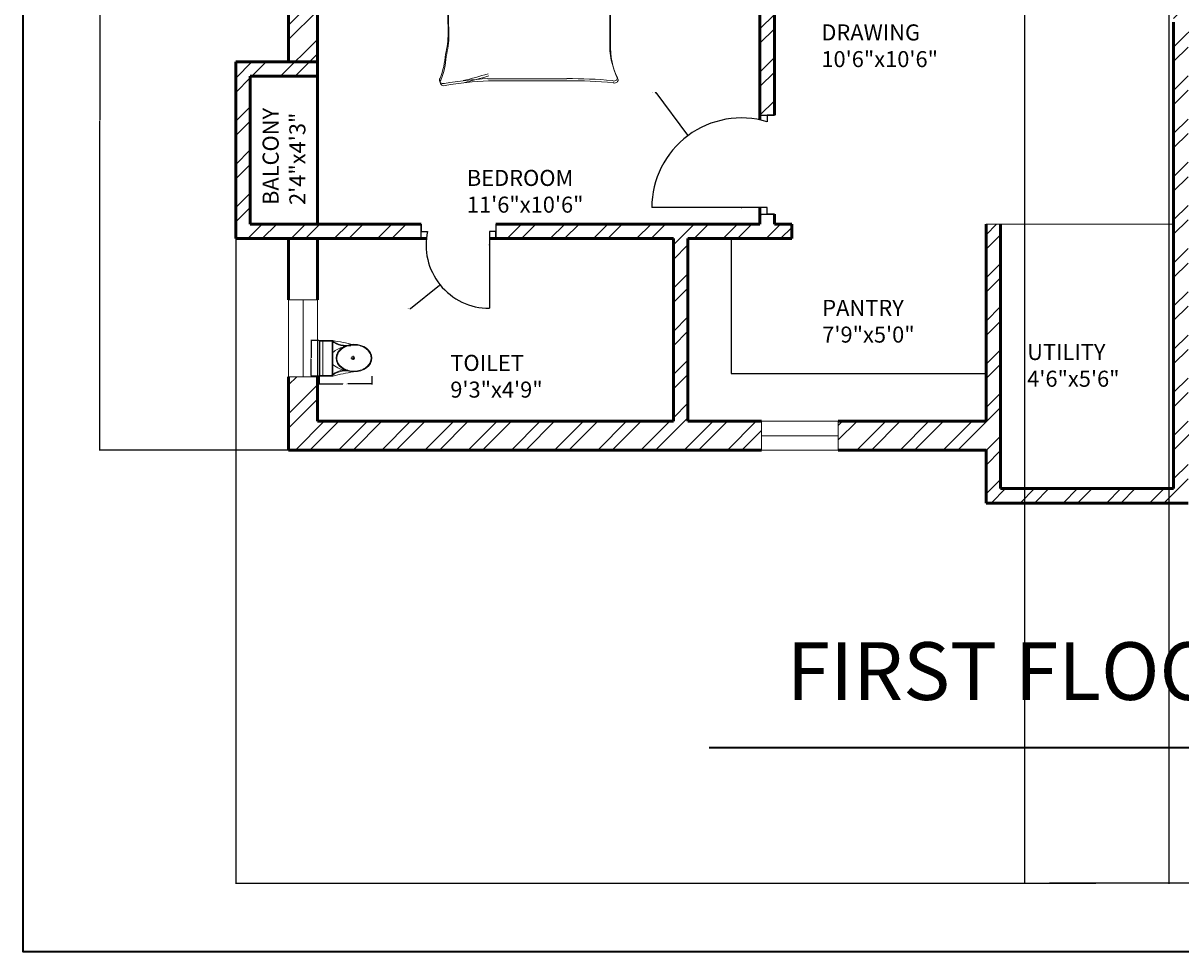
# Model space of a CAD drawing. Units: inches. Extents: x 1896 to 2572, y 1528 to 2474.
# Tile 1 of 10: x 1896 to 2257, y 1528 to 1818. Entities that reach past the tile are written whole.
import ezdxf

# ---------------------------------------------------------------- set-up
doc = ezdxf.new("R2010")
doc.units = ezdxf.units.IN
for name, color, linetype, lineweight in [('A-ANNO-DIMS', 2, 'Continuous', 18), ('A-ANNO-TTLB', 7, 'Continuous', 35), ('A-AREA-IDEN', 7, 'Continuous', 18), ('A-DOOR', 11, 'Continuous', 25), ('A-FLOR', 7, 'Continuous', 18), ('A-FLOR-CASE', 7, 'Continuous', 25), ('A-FLOR-FIXT', 8, 'Continuous', 18), ('A-FURN', 8, 'Continuous', 18), ('A-GLAZ', 131, 'Continuous', 20), ('A-WALL', 7, 'Continuous', 50)]:
    doc.layers.add(name, color=color, linetype=linetype, lineweight=lineweight)
doc.layers.add('A-WALL-PATT', color=215, linetype='Continuous', lineweight=13, true_color=0xa953a0)
doc.styles.get("Standard").update_dxf_attribs({"font": 'arial.ttf'})
doc.dimstyles.get("Standard").update_dxf_attribs({"dimtxt": 0.18, "dimasz": 0.18, "dimexe": 0.18, "dimexo": 0.0625, "dimgap": 0.09, "dimtad": 0, "dimtih": 1, "dimtoh": 1, "dimdec": 4, "dimzin": 0, "dimdsep": 46, "dimtxsty": 'Standard', "dimcen": 0.09, "dimadec": 0, "dimazin": 0, "dimtfac": 1, "dimtdec": 4, "dimtofl": 0, "dimtmove": 0, "dimatfit": 3, "dimfxl": 1, "dimtolj": 1, "dimtzin": 0, "dimarcsym": 0})

# ---------------------------------------------------------------- blocks, each defined once
blk = doc.blocks.new('A$C31115884')
for p, q in [((258, 466), (258, 523)), ((283, 498), (223, 498)), ((0, 200), (0, 0)), ((520, 200), (0, 200)), ((10, 190), (10, 10)), ((510, 190), (10, 190)), ((510, 10), (510, 190)), ((520, 0), (520, 200)), ((510, 54), (0, 54)), ((10, 10), (510, 10)), ((0, 0), (520, 0))]:
    blk.add_line(p, q)
blk.add_circle((256, 496), 23.6)
for centre, radius, start, end in [((2778, -205), 2807, 165.4549, 171.7133), ((-295, 403), 365, 324.2091, 9.3499), ((-295, 403), 375, 324.2091, 9.3499), ((384, 406), 293, 190.2774, 224.1564), ((139, 406), 293, 315.8436, 2.6563), ((806, 403), 375, 179.2036, 215.7909), ((806, 403), 365, 170.6501, 215.7909), ((3237, 905), 2807, 188.2867, 194.5451)]:
    blk.add_arc(centre, radius, start, end)
blk.add_ellipse((256, 510), major_axis=(0, -261), ratio=0.772727)
blk.add_open_spline([(256, 259), (263, 259), (270, 260), (288, 262), (299, 265), (320, 273), (330, 278), (350, 291), (360, 299), (378, 316), (386, 326), (402, 347), (409, 358), (421, 383), (427, 395), (436, 422), (440, 436), (445, 465), (447, 480), (448, 509), (448, 524), (445, 553), (443, 568), (436, 596), (432, 610), (422, 636), (416, 649), (402, 672), (395, 683), (379, 703), (370, 712), (351, 728), (341, 735), (321, 746), (310, 751), (289, 757), (278, 759), (256, 761), (245, 761), (223, 757), (212, 754), (191, 746), (181, 741), (161, 728), (151, 720), (133, 703), (125, 693), (110, 672), (103, 660), (90, 636), (85, 623), (76, 596), (72, 582), (67, 553), (66, 538), (64, 509), (65, 494), (68, 465), (70, 450), (77, 422), (81, 408), (91, 382), (97, 370), (111, 346), (118, 335), (135, 316), (144, 307), (162, 291), (172, 284), (193, 273), (203, 269), (225, 262), (236, 260), (250, 259), (253, 259), (256, 259)], degree=3, knots=[0, 0, 0, 0, 0.110105, 0.110105, 0.285049, 0.285049, 0.459994, 0.459994, 0.634938, 0.634938, 0.809882, 0.809882, 0.984827, 0.984827, 1.159771, 1.159771, 1.334715, 1.334715, 1.50966, 1.50966, 1.684604, 1.684604, 1.859549, 1.859549, 2.034493, 2.034493, 2.209437, 2.209437, 2.384382, 2.384382, 2.559326, 2.559326, 2.73427, 2.73427, 2.909215, 2.909215, 3.084159, 3.084159, 3.259103, 3.259103, 3.434048, 3.434048, 3.608992, 3.608992, 3.783936, 3.783936, 3.958881, 3.958881, 4.133825, 4.133825, 4.30877, 4.30877, 4.483714, 4.483714, 4.658658, 4.658658, 4.833603, 4.833603, 5.008547, 5.008547, 5.183491, 5.183491, 5.358436, 5.358436, 5.53338, 5.53338, 5.708324, 5.708324, 5.883269, 5.883269, 6.058213, 6.058213, 6.233158, 6.233158, 6.283185, 6.283185, 6.283185, 6.283185])
blk = doc.blocks.new('BED-DOUBLE')
for p, q in [((3.47, 63.33), (3.47, 81.44)), ((3.47, 63.33), (3.47, 81.44)), ((3.47, 81.44), (51.49, 81.44)), ((3.47, 79.91), (51.27, 79.91)), ((3.47, 79.91), (51.26, 79.91)), ((3.7, 62.69), (3.7, 80.8)), ((3.7, 62.69), (3.7, 80.8)), ((24.54, 78.99), (25.98, 79.57)), ((24.54, 78.99), (25.98, 79.57)), ((25.98, 79.57), (26.56, 74.22)), ((25.98, 79.57), (26.56, 74.22)), ((51.26, 81.44), (51.26, 54.83)), ((51.27, 81.44), (51.27, 54.83)), ((51.49, 81.44), (51.49, 80.8)), ((51.49, 80.8), (51.49, 54.19)), ((51.49, 80.8), (51.49, 54.19)), ((3.7, 79.27), (51.49, 79.27)), ((3.7, 79.27), (51.49, 79.27)), ((3.89, 78.13), (4.47, 74.95)), ((3.89, 78.13), (4.47, 74.95)), ((3.9, 78.11), (8.18, 78.43)), ((3.9, 78.11), (8.18, 78.43)), ((4.12, 77.49), (4.7, 74.31)), ((4.12, 77.49), (4.7, 74.31)), ((4.13, 77.47), (8.41, 77.8)), ((4.13, 77.47), (8.41, 77.8)), ((8.18, 78.43), (8.28, 78.42)), ((8.18, 78.43), (8.28, 78.42)), ((8.28, 78.42), (12.11, 78.13)), ((8.28, 78.42), (12.11, 78.13)), ((8.41, 77.8), (8.51, 77.78)), ((8.41, 77.8), (8.51, 77.78)), ((8.51, 77.78), (12.34, 77.49)), ((8.51, 77.78), (12.34, 77.49)), ((12.11, 78.13), (17.6, 77.12)), ((12.11, 78.13), (17.6, 77.12)), ((12.34, 77.49), (17.83, 76.48)), ((12.34, 77.49), (17.83, 76.48)), ((14.85, 77.69), (16.88, 78.42)), ((14.85, 77.69), (16.88, 78.42)), ((15.08, 77.05), (17.11, 77.78)), ((15.08, 77.05), (17.11, 77.78)), ((16.88, 78.42), (19.77, 79.14)), ((16.88, 78.42), (19.77, 79.14)), ((17.11, 77.78), (20, 78.5)), ((17.11, 77.78), (20, 78.5)), ((19.77, 79.14), (20.09, 79.14)), ((19.77, 79.14), (20.09, 79.14)), ((20, 78.5), (20.32, 78.5)), ((20, 78.5), (20.32, 78.5)), ((20.09, 79.14), (24.54, 78.99)), ((20.09, 79.14), (24.54, 78.99)), ((20.32, 78.5), (24.77, 78.36)), ((20.32, 78.5), (24.76, 78.36)), ((24.76, 78.36), (26.21, 78.93)), ((24.77, 78.36), (26.21, 78.93)), ((26.21, 78.93), (26.79, 73.58)), ((26.21, 78.93), (26.79, 73.58)), ((27.98, 78.95), (27.73, 73.58)), ((27.98, 78.95), (27.73, 73.58)), ((28.21, 78.31), (27.96, 72.94)), ((28.2, 78.31), (27.96, 72.94)), ((29.46, 78.46), (27.98, 78.95)), ((29.46, 78.46), (27.98, 78.95)), ((29.68, 77.83), (28.2, 78.31)), ((29.68, 77.83), (28.21, 78.31)), ((33.88, 78.89), (29.46, 78.46)), ((33.88, 78.89), (29.46, 78.46)), ((34.11, 78.25), (29.68, 77.83)), ((34.11, 78.25), (29.68, 77.83)), ((34.2, 78.91), (33.88, 78.89)), ((34.2, 78.91), (33.88, 78.89)), ((34.43, 78.27), (34.11, 78.25)), ((34.43, 78.27), (34.11, 78.25)), ((37.14, 78.37), (34.2, 78.91)), ((37.13, 78.37), (34.2, 78.91)), ((37.36, 77.73), (34.43, 78.27)), ((37.36, 77.73), (34.43, 78.27)), ((41.91, 78.37), (36.49, 77.02)), ((41.91, 78.37), (36.49, 77.02)), ((42.14, 77.73), (36.72, 76.38)), ((42.14, 77.73), (36.72, 76.38)), ((39.2, 77.77), (37.13, 78.37)), ((39.2, 77.77), (37.14, 78.37)), ((39.43, 77.13), (37.36, 77.73)), ((39.43, 77.13), (37.36, 77.73)), ((45.71, 78.9), (41.91, 78.37)), ((45.71, 78.9), (41.91, 78.37)), ((45.94, 78.26), (42.14, 77.73)), ((45.94, 78.26), (42.14, 77.73)), ((50.11, 78.89), (44.71, 78.98)), ((44.71, 78.98), (45.71, 78.9)), ((50.11, 78.89), (44.71, 78.98)), ((44.71, 78.98), (45.71, 78.9)), ((50.34, 78.25), (44.94, 78.34)), ((44.94, 78.34), (45.94, 78.26)), ((50.34, 78.25), (44.94, 78.34)), ((44.94, 78.34), (45.94, 78.26)), ((49.31, 73.19), (48.13, 75.87)), ((49.31, 73.19), (48.13, 75.87)), ((50.11, 78.89), (49.73, 75.68)), ((50.11, 78.89), (49.73, 75.68)), ((50.34, 78.25), (49.96, 75.04)), ((50.34, 78.25), (49.96, 75.04)), ((4.47, 74.95), (4.04, 72.34)), ((4.47, 74.95), (4.04, 72.34)), ((4.04, 72.34), (4.62, 71.33)), ((4.04, 72.34), (4.62, 71.33)), ((4.7, 74.31), (4.27, 71.7)), ((4.7, 74.31), (4.27, 71.7)), ((4.47, 68.87), (5.05, 72.49)), ((4.47, 68.87), (5.05, 72.49)), ((5.05, 72.49), (6.06, 75.24)), ((5.05, 72.49), (6.06, 75.24)), ((5.28, 71.85), (6.29, 74.6)), ((5.28, 71.85), (6.29, 74.6)), ((26.56, 74.22), (27.14, 71.04)), ((26.56, 74.22), (27.14, 71.04)), ((26.79, 73.58), (27.37, 70.4)), ((26.79, 73.58), (27.37, 70.4)), ((27.73, 73.58), (27.35, 70.37)), ((27.73, 73.58), (27.35, 70.37)), ((27.96, 72.94), (27.58, 69.73)), ((27.96, 72.94), (27.58, 69.73)), ((49.54, 72.55), (48.36, 75.23)), ((49.54, 72.55), (48.36, 75.23)), ((50.11, 69.61), (49.31, 73.19)), ((50.11, 69.61), (49.31, 73.19)), ((50.34, 68.98), (49.54, 72.55)), ((50.34, 68.98), (49.54, 72.55)), ((49.73, 75.68), (50.33, 73.11)), ((49.73, 75.68), (50.33, 73.11)), ((50.33, 73.11), (49.81, 72.06)), ((50.33, 73.11), (49.81, 72.06)), ((49.96, 75.04), (50.56, 72.47)), ((49.96, 75.04), (50.56, 72.47)), ((50.56, 72.47), (50.04, 71.42)), ((50.56, 72.47), (50.04, 71.42)), ((4.27, 71.7), (4.85, 70.69)), ((4.27, 71.7), (4.85, 70.69)), ((4.76, 67.28), (4.47, 68.87)), ((4.76, 67.28), (4.47, 68.87)), ((4.7, 68.23), (5.28, 71.85)), ((4.7, 68.23), (5.28, 71.85)), ((27.14, 69.74), (26.56, 67.86)), ((27.14, 69.74), (26.56, 67.86)), ((27.37, 69.1), (26.79, 67.22)), ((27.37, 69.1), (26.79, 67.22)), ((27.14, 71.04), (27.14, 69.74)), ((27.14, 71.04), (27.14, 69.74)), ((27.35, 70.37), (27.44, 69.07)), ((27.35, 70.37), (27.44, 69.07)), ((27.37, 70.4), (27.37, 69.1)), ((27.37, 70.4), (27.37, 69.1)), ((27.44, 69.07), (28.13, 67.23)), ((27.44, 69.07), (28.13, 67.23)), ((27.58, 69.73), (27.66, 68.43)), ((27.58, 69.73), (27.66, 68.43)), ((49.92, 68.01), (50.11, 69.61)), ((49.92, 68.01), (50.11, 69.61)), ((50.15, 67.37), (50.34, 68.98)), ((50.15, 67.37), (50.34, 68.98)), ((4.18, 64.1), (4.76, 67.28)), ((4.18, 64.1), (4.76, 67.28)), ((4.41, 63.46), (4.99, 66.64)), ((4.41, 63.46), (4.99, 66.64)), ((4.99, 66.64), (4.7, 68.23)), ((4.99, 66.64), (4.7, 68.23)), ((6.38, 65.81), (10.41, 65.15)), ((6.38, 65.81), (10.41, 65.15)), ((6.61, 65.18), (10.64, 64.51)), ((6.61, 65.18), (10.64, 64.51)), ((10.41, 65.15), (9.28, 64.83)), ((10.41, 65.15), (9.28, 64.83)), ((10.41, 65.15), (17.42, 64.72)), ((10.41, 65.15), (17.42, 64.72)), ((17.42, 64.72), (19.38, 65.27)), ((17.42, 64.72), (19.38, 65.27)), ((19.38, 65.27), (24.52, 64.87)), ((19.38, 65.27), (24.52, 64.87)), ((24.1, 65.18), (20.96, 66.27)), ((24.1, 65.18), (20.96, 66.27)), ((24.33, 64.54), (21.19, 65.63)), ((24.33, 64.54), (21.19, 65.63)), ((26.56, 65.18), (24.1, 65.18)), ((26.56, 65.18), (24.1, 65.18)), ((26.56, 67.86), (26.56, 65.18)), ((26.56, 67.86), (26.56, 65.18)), ((26.79, 67.22), (26.79, 64.54)), ((26.79, 67.22), (26.79, 64.54)), ((27.66, 68.43), (28.36, 66.59)), ((27.66, 68.43), (28.36, 66.59)), ((28.13, 67.23), (28.3, 64.55)), ((28.13, 67.23), (28.3, 64.55)), ((28.36, 66.59), (28.53, 63.91)), ((28.36, 66.59), (28.53, 63.91)), ((30.75, 64.7), (33.82, 65.99)), ((30.75, 64.7), (33.82, 65.99)), ((30.98, 64.06), (34.05, 65.35)), ((30.98, 64.06), (34.05, 65.35)), ((32.56, 65.81), (36.6, 65.15)), ((32.56, 65.81), (36.6, 65.15)), ((32.79, 65.18), (36.82, 64.51)), ((32.79, 65.18), (36.82, 64.51)), ((36.6, 65.15), (43.61, 64.72)), ((36.6, 65.15), (43.61, 64.72)), ((43.61, 64.72), (45.57, 65.27)), ((43.61, 64.72), (45.57, 65.27)), ((45.57, 65.27), (50.7, 64.87)), ((45.57, 65.27), (50.7, 64.87)), ((50.7, 64.87), (49.92, 68.01)), ((50.7, 64.87), (49.92, 68.01)), ((50.93, 64.23), (50.15, 67.37)), ((50.93, 64.23), (50.15, 67.37)), ((9.28, 64.83), (4.18, 64.1)), ((9.28, 64.83), (4.18, 64.1)), ((9.51, 64.19), (4.41, 63.46)), ((9.51, 64.19), (4.41, 63.46)), ((10.64, 64.51), (9.51, 64.19)), ((10.64, 64.51), (9.51, 64.19)), ((10.64, 64.51), (17.65, 64.08)), ((10.64, 64.51), (17.65, 64.08)), ((17.65, 64.08), (19.61, 64.63)), ((17.65, 64.08), (19.61, 64.63)), ((19.61, 64.63), (24.74, 64.23)), ((19.61, 64.63), (24.74, 64.23)), ((26.79, 64.54), (24.33, 64.54)), ((26.79, 64.54), (24.33, 64.54)), ((28.3, 64.55), (30.75, 64.7)), ((28.3, 64.55), (30.75, 64.7)), ((28.53, 63.91), (30.98, 64.06)), ((28.53, 63.91), (30.98, 64.06)), ((30.26, 64.06), (34.45, 57.57)), ((30.26, 64.06), (34.45, 57.57)), ((30.49, 63.42), (34.68, 56.93)), ((30.49, 63.42), (34.68, 56.93)), ((40.64, 61.13), (32.31, 64.06)), ((40.64, 61.13), (32.31, 64.06)), ((40.87, 60.49), (32.53, 63.42)), ((40.87, 60.49), (32.53, 63.42)), ((36.82, 64.51), (43.83, 64.08)), ((36.82, 64.51), (43.83, 64.08)), ((43.83, 64.08), (45.79, 64.63)), ((43.83, 64.08), (45.79, 64.63)), ((45.79, 64.63), (50.93, 64.23)), ((45.79, 64.63), (50.93, 64.23)), ((46.22, 59.11), (40.64, 61.13)), ((46.22, 59.11), (40.64, 61.13)), ((46.45, 58.48), (40.87, 60.49)), ((46.45, 58.48), (40.87, 60.49)), ((49.16, 56.95), (46.22, 59.11)), ((49.16, 56.95), (46.22, 59.11)), ((49.39, 56.31), (46.45, 58.48)), ((49.39, 56.31), (46.45, 58.48)), ((34.45, 57.57), (36.15, 53.08)), ((34.45, 57.57), (36.15, 53.08)), ((34.68, 56.93), (36.38, 52.44)), ((34.68, 56.93), (36.38, 52.44)), ((52.87, 53.7), (49.16, 56.95)), ((52.87, 53.7), (49.16, 56.95)), ((53.1, 53.06), (49.39, 56.31)), ((53.1, 53.06), (49.39, 56.31)), ((36.15, 53.08), (36.46, 51.07)), ((36.15, 53.08), (36.46, 51.07)), ((36.38, 52.44), (36.69, 50.43)), ((36.38, 52.44), (36.69, 50.43)), ((36.46, 51.07), (38.94, 51.69)), ((36.46, 51.07), (38.94, 51.69)), ((36.69, 50.43), (39.17, 51.05)), ((36.69, 50.43), (39.17, 51.05)), ((38.94, 51.69), (40.95, 52.61)), ((38.94, 51.69), (40.95, 52.61)), ((39.17, 51.05), (41.18, 51.97)), ((39.17, 51.05), (41.18, 51.97)), ((40.95, 52.61), (44.36, 53.08)), ((40.95, 52.61), (44.36, 53.08)), ((41.18, 51.97), (44.59, 52.44)), ((41.18, 51.97), (44.59, 52.44)), ((44.36, 53.08), (48.23, 53.39)), ((44.36, 53.08), (48.23, 53.39)), ((44.59, 52.44), (48.46, 52.75)), ((44.59, 52.44), (48.46, 52.75)), ((48.23, 53.39), (51.33, 53.08)), ((48.23, 53.39), (51.33, 53.08)), ((48.46, 52.75), (51.56, 52.44)), ((48.46, 52.75), (51.56, 52.44)), ((51.33, 53.08), (52.87, 53.7)), ((51.33, 53.08), (52.87, 53.7)), ((51.56, 52.44), (53.1, 53.06)), ((51.56, 52.44), (53.1, 53.06)), ((52.95, 51.95), (52.87, 53.7, 3.87)), ((52.95, 51.95), (52.87, 53.7, 3.87)), ((53.18, 51.31), (53.1, 53.06, 3.87)), ((53.17, 51.31), (53.1, 53.06, 3.87)), ((15.06, 2.2), (39.68, 2.2)), ((15.06, 2.2), (39.68, 2.2)), ((15.29, 1.56), (39.91, 1.56)), ((15.29, 1.56), (39.91, 1.56))]:
    blk.add_line(p, q)
for centre, radius, start, end in [((85.16, 61.35), 83.31, 178.7218, 185.604), ((85.16, 61.35), 83.31, 178.7218, 185.604), ((21.36, -100.61), 164.97, 86.0865, 96.7821), ((21.36, -100.61), 164.97, 86.0865, 96.7821), ((85.39, 60.71), 83.31, 178.7218, 185.604), ((85.39, 60.71), 83.31, 178.7218, 185.604), ((21.59, -101.25), 164.97, 86.0865, 96.7821), ((21.59, -101.25), 164.97, 86.0865, 96.7821), ((17.76, -74.87), 129.02, 81.7845, 96.9006), ((17.76, -74.87), 129.02, 81.7845, 96.9006), ((17.98, -75.51), 129.02, 81.7845, 96.9006), ((17.98, -75.51), 129.02, 81.7845, 96.9006), ((-167.31, 50.27), 170.11, 358.4762, 1.0082), ((-167.31, 50.27), 170.11, 358.4762, 1.0082), ((-167.08, 49.63), 170.11, 358.4762, 1.0082), ((-167.08, 49.63), 170.11, 358.4762, 1.0082), ((36.64, 51), 0.185, 160.2464, 271.1377), ((36.64, 51), 0.185, 160.2464, 271.1377), ((31.15, 79.96), 29.65, 280.6617, 289.8806), ((31.15, 79.96), 29.65, 280.6617, 289.8806), ((31.38, 79.32), 29.65, 280.6617, 289.8806), ((31.38, 79.32), 29.65, 280.6617, 289.8806), ((43.74, 46.38), 6.22, 78.6608, 113.7384), ((43.74, 46.38), 6.22, 78.6608, 113.7384), ((43.97, 45.74), 6.22, 78.6608, 113.7384), ((43.97, 45.74), 6.22, 78.6608, 113.7384), ((51.33, 88.1), 36.18, 259.8763, 272.5657), ((51.33, 88.1), 36.18, 259.8763, 272.5657), ((51.56, 87.46), 36.18, 259.8763, 272.5657), ((51.56, 87.46), 36.18, 259.8763, 272.5657), ((182.27, 45.13), 129.5, 176.9791, 183.8365), ((182.27, 45.13), 129.5, 176.9791, 183.8365), ((182.49, 44.49), 129.5, 176.9791, 183.8365), ((182.49, 44.49), 129.5, 176.9791, 183.8365), ((36.86, 50.36), 0.185, 160.2464, 271.1377), ((36.86, 50.36), 0.185, 160.2464, 271.1377), ((484.82, 30.83), 482.31, 178.2277, 181.7185), ((484.82, 30.83), 482.31, 178.2277, 181.7185), ((485.05, 30.19), 482.31, 178.2277, 181.7185), ((485.05, 30.19), 482.31, 178.2277, 181.7185), ((-4508.74, 13.62), 4561.86, 0.00217, 0.28689), ((-4508.74, 13.62), 4561.86, 0.00217, 0.28689), ((-4508.52, 12.98), 4561.86, 0.00217, 0.28689), ((-4508.52, 12.98), 4561.86, 0.00217, 0.28689), ((-26.9, 16.93), 29.63, 346.0648, 358.9113), ((-26.9, 16.93), 29.63, 346.0648, 358.9113), ((-26.67, 16.29), 29.63, 346.0648, 358.9113), ((-26.67, 16.29), 29.63, 346.0648, 358.9113), ((76.16, 12.78), 23.07, 177.4714, 206.4681), ((76.16, 12.78), 23.07, 177.4714, 206.4681), ((76.39, 12.14), 23.07, 177.4714, 206.4681), ((76.39, 12.14), 23.07, 177.4714, 206.4681), ((-21.66, 11.17), 23.56, 337.9751, 356.652), ((-21.66, 11.17), 23.56, 337.9751, 356.652), ((-21.43, 10.53), 23.56, 337.9751, 356.652), ((-21.43, 10.53), 23.56, 337.9751, 356.652), ((-17.22, 105.16), 106.46, 283.3832, 287.7053), ((-17.22, 105.16), 106.46, 283.3832, 287.7053), ((1.09, 1.73), 1.09, 146.1736, 293.4781), ((1.09, 1.73), 1.09, 146.1736, 293.4781), ((1.32, 1.09), 1.09, 146.1736, 293.4781), ((1.32, 1.09), 1.09, 146.1736, 293.4781), ((21.43, -119.39), 121.76, 92.9958, 99.4091), ((21.43, -119.39), 121.76, 92.9958, 99.4091), ((21.65, -120.03), 121.76, 92.9958, 99.4091), ((21.65, -120.03), 121.76, 92.9958, 99.4091), ((-16.99, 104.52), 106.46, 283.3832, 287.7053), ((-16.99, 104.52), 106.46, 283.3832, 287.7053), ((41.15, -130.83), 133.04, 84.4998, 90.6351), ((41.15, -130.83), 133.04, 84.4998, 90.6351), ((41.38, -131.47), 133.04, 84.4998, 90.6351), ((41.38, -131.47), 133.04, 84.4998, 90.6351), ((54.41, 2.57), 1.1, 242.6588, 356.02), ((54.41, 2.57), 1.1, 242.6588, 356.02), ((54.64, 1.93), 1.1, 242.6588, 356.02), ((54.64, 1.93), 1.1, 242.6588, 356.02)]:
    blk.add_arc(centre, radius, start, end)
blk = doc.blocks.new('WIN-24IN')
for p, q in [((4.5, 24), (0, 24)), ((0, 24), (9, 24)), ((0, 24), (0, 0)), ((4.5, 0), (4.5, 24)), ((9, 0), (9, 24)), ((0, 0), (9, 0)), ((9, 0), (4.5, 0))]:
    blk.add_line(p, q)
blk = doc.blocks.new('*D9')
at = {"layer": 'A-ANNO-DIMS', "color": 0, "lineweight": -2, "transparency": 16777216}
for p, q in [((1988.15, 1707.44), (1988.15, 1704.86)), ((1988.33, 1705.04), (1995.58, 1705.04)), ((2004.37, 1705.04), (1997.13, 1705.04)), ((2004.55, 1707.44), (2004.55, 1704.86))]:
    blk.add_line(p, q, dxfattribs=at)
at = {"layer": 'A-ANNO-DIMS', "color": 0, "transparency": 16777216}
for points in [[(1988.33, 1705.07), (1988.33, 1705.01), (1988.15, 1705.04)], [(2004.37, 1705.07), (2004.37, 1705.01), (2004.55, 1705.04)]]:
    blk.add_solid(points, dxfattribs=at)
at = {"layer": 'Defpoints', "color": 0, "transparency": 16777216}
for p in [(1988.15, 1707.5), (2004.55, 1707.5), (2004.55, 1705.04)]:
    blk.add_point(p, dxfattribs=at)
at = {"layer": 'A-ANNO-DIMS', "color": 0, "transparency": 16777216, "insert": (1996.35, 1705.04), "char_height": 0.18, "attachment_point": 5}
blk.add_mtext('\\A1;WC 16 TYP.', dxfattribs=at)
blk = doc.blocks.new('*D10')
at = {"layer": 'A-ANNO-DIMS', "color": 0, "lineweight": -2, "transparency": 16777216}
for p, q in [((1988.09, 1718.57), (1985.51, 1718.57)), ((1985.69, 1718.39), (1985.69, 1713.22)), ((1985.69, 1707.68), (1985.69, 1712.86)), ((1988.09, 1707.5), (1985.51, 1707.5))]:
    blk.add_line(p, q, dxfattribs=at)
at = {"layer": 'A-ANNO-DIMS', "color": 0, "transparency": 16777216}
for points in [[(1985.66, 1718.39), (1985.72, 1718.39), (1985.69, 1718.57)], [(1985.66, 1707.68), (1985.72, 1707.68), (1985.69, 1707.5)]]:
    blk.add_solid(points, dxfattribs=at)
at = {"layer": 'Defpoints', "color": 0, "transparency": 16777216}
for p in [(1988.15, 1718.57), (1985.69, 1707.5), (1988.15, 1707.5)]:
    blk.add_point(p, dxfattribs=at)
at = {"layer": 'A-ANNO-DIMS', "color": 0, "transparency": 16777216, "insert": (1985.69, 1713.04), "char_height": 0.18, "attachment_point": 5}
blk.add_mtext('\\A1;11 TYP.', dxfattribs=at)
blk = doc.blocks.new('*D19')
at = {"layer": 'A-ANNO-DIMS', "color": 0, "lineweight": -2, "transparency": 16777216}
for p, q in [((2469.12, 1813.34), (2469.12, 1549.1)), ((1962.12, 1750.34), (1962.12, 1549.1)), ((1962.3, 1549.28), (2215.33, 1549.28)), ((2468.94, 1549.28), (2215.91, 1549.28))]:
    blk.add_line(p, q, dxfattribs=at)
at = {"layer": 'A-ANNO-DIMS', "color": 0, "transparency": 16777216}
for points in [[(1962.3, 1549.31), (1962.3, 1549.25), (1962.12, 1549.28)], [(2468.94, 1549.31), (2468.94, 1549.25), (2469.12, 1549.28)]]:
    blk.add_solid(points, dxfattribs=at)
at = {"layer": 'Defpoints', "color": 0, "transparency": 16777216}
for p in [(2469.12, 1813.4), (1962.12, 1750.4), (2469.12, 1549.28)]:
    blk.add_point(p, dxfattribs=at)
at = {"layer": 'A-ANNO-DIMS', "color": 0, "transparency": 16777216, "insert": (2215.62, 1549.28), "char_height": 0.18, "attachment_point": 5}
blk.add_mtext('\\A1;507', dxfattribs=at)
blk = doc.blocks.new('*D20')
at = {"layer": 'A-ANNO-DIMS', "color": 0, "lineweight": -2, "transparency": 16777216}
for p, q in [((2180.68, 2431.4), (2511.65, 2431.4)), ((2511.47, 2431.22), (2511.47, 2049.83)), ((2511.47, 1668.08), (2511.47, 2049.47)), ((2452.68, 1667.9), (2511.65, 1667.9))]:
    blk.add_line(p, q, dxfattribs=at)
at = {"layer": 'A-ANNO-DIMS', "color": 0, "transparency": 16777216}
for points in [[(2511.44, 2431.22), (2511.5, 2431.22), (2511.47, 2431.4)], [(2511.44, 1668.08), (2511.5, 1668.08), (2511.47, 1667.9)]]:
    blk.add_solid(points, dxfattribs=at)
at = {"layer": 'Defpoints', "color": 0, "transparency": 16777216}
for p in [(2180.62, 2431.4), (2511.47, 2431.4), (2452.62, 1667.9)]:
    blk.add_point(p, dxfattribs=at)
at = {"layer": 'A-ANNO-DIMS', "color": 0, "transparency": 16777216, "insert": (2511.47, 2049.65), "char_height": 0.18, "attachment_point": 5}
blk.add_mtext('\\A1;763.5', dxfattribs=at)
blk = doc.blocks.new('*D28')
at = {"layer": 'A-ANNO-DIMS', "color": 0, "lineweight": -2, "transparency": 16777216}
for p, q in [((1987.56, 1889.9), (1919.59, 1889.9)), ((1919.77, 1889.72), (1919.77, 1787.33)), ((1919.77, 1684.58), (1919.77, 1786.97)), ((1978.56, 1684.4), (1919.59, 1684.4))]:
    blk.add_line(p, q, dxfattribs=at)
at = {"layer": 'A-ANNO-DIMS', "color": 0, "transparency": 16777216}
for points in [[(1919.74, 1889.72), (1919.8, 1889.72), (1919.77, 1889.9)], [(1919.74, 1684.58), (1919.8, 1684.58), (1919.77, 1684.4)]]:
    blk.add_solid(points, dxfattribs=at)
at = {"layer": 'Defpoints', "color": 0, "transparency": 16777216}
for p in [(1987.62, 1889.9), (1919.77, 1684.4), (1978.62, 1684.4)]:
    blk.add_point(p, dxfattribs=at)
at = {"layer": 'A-ANNO-DIMS', "color": 0, "transparency": 16777216, "insert": (1919.77, 1787.15), "char_height": 0.18, "attachment_point": 5}
blk.add_mtext('\\A1;205.5', dxfattribs=at)
blk = doc.blocks.new('*D33')
at = {"layer": 'A-ANNO-DIMS', "color": 0, "lineweight": -2, "transparency": 16777216}
for p, q in [((2208.12, 2166.84), (2208.12, 1549.1)), ((2253.12, 2166.84), (2253.12, 1549.1)), ((2208.3, 1549.28), (2230.4, 1549.28)), ((2252.94, 1549.28), (2230.85, 1549.28))]:
    blk.add_line(p, q, dxfattribs=at)
at = {"layer": 'A-ANNO-DIMS', "color": 0, "transparency": 16777216}
for points in [[(2208.3, 1549.31), (2208.3, 1549.25), (2208.12, 1549.28)], [(2252.94, 1549.31), (2252.94, 1549.25), (2253.12, 1549.28)]]:
    blk.add_solid(points, dxfattribs=at)
at = {"layer": 'Defpoints', "color": 0, "transparency": 16777216}
for p in [(2208.12, 2166.9), (2253.12, 2166.9), (2253.12, 1549.28)]:
    blk.add_point(p, dxfattribs=at)
at = {"layer": 'A-ANNO-DIMS', "color": 0, "transparency": 16777216, "insert": (2230.62, 1549.28), "char_height": 0.18, "attachment_point": 5}
blk.add_mtext('\\A1;45', dxfattribs=at)
blk = doc.blocks.new('*D39')
at = {"layer": 'A-ANNO-DIMS', "color": 0, "lineweight": -2, "transparency": 16777216}
for p, q in [((2092.94, 1795.95), (2093.12, 1795.95)), ((2093.12, 1795.95), (2103.04, 1782.64)), ((2119.75, 1760.05), (2119.93, 1760.05)), ((2119.84, 1759.96), (2119.84, 1760.14))]:
    blk.add_line(p, q, dxfattribs=at)
at = {"layer": 'A-ANNO-DIMS', "color": 0, "transparency": 16777216}
blk.add_solid([(2103.06, 1782.65), (2103.01, 1782.62), (2103.14, 1782.49)], dxfattribs=at)
at = {"layer": 'Defpoints', "color": 0, "transparency": 16777216}
for p in [(2103.14, 1782.49), (2119.84, 1760.05)]:
    blk.add_point(p, dxfattribs=at)
at = {"layer": 'A-ANNO-DIMS', "color": 0, "transparency": 16777216, "insert": (2092.46, 1795.95), "char_height": 0.18, "attachment_point": 5}
blk.add_mtext('\\A1;R27.97', dxfattribs=at)
blk = doc.blocks.new('*D46')
at = {"layer": 'A-ANNO-DIMS', "color": 0, "lineweight": -2, "transparency": 16777216}
for p, q in [((2041.14, 1748.41), (2041.32, 1748.41)), ((2041.23, 1748.32), (2041.23, 1748.5)), ((2016.59, 1728.6), (2025.69, 1735.91)), ((2016.41, 1728.6), (2016.59, 1728.6))]:
    blk.add_line(p, q, dxfattribs=at)
at = {"layer": 'A-ANNO-DIMS', "color": 0, "transparency": 16777216}
blk.add_solid([(2025.67, 1735.94), (2025.71, 1735.89), (2025.83, 1736.02)], dxfattribs=at)
at = {"layer": 'Defpoints', "color": 0, "transparency": 16777216}
for p in [(2041.23, 1748.41), (2025.83, 1736.02)]:
    blk.add_point(p, dxfattribs=at)
at = {"layer": 'A-ANNO-DIMS', "color": 0, "transparency": 16777216, "insert": (2015.93, 1728.6), "char_height": 0.18, "attachment_point": 5}
blk.add_mtext('\\A1;R19.76', dxfattribs=at)

msp = doc.modelspace()

# ---------------------------------------------------------------- hatches: boundary and pattern name
at = {"layer": 'A-WALL-PATT'}
h = msp.add_hatch(dxfattribs=at)
h.set_pattern_fill('ANSI32', color=256)
h.paths.add_polyline_path([(2071.6224, 2382.3979), (2071.6224, 2422.3979), (2110.6224, 2422.3979), (2110.6224, 2382.3979), (2110.6224, 2357.5961), (2119.6224, 2357.5961), (2119.6224, 2422.3979), (2171.6224, 2422.3979), (2171.6224, 2373.3979), (2193.5093, 2373.3979), (2193.5093, 2377.8979), (2193.5093, 2382.3979), (2180.6224, 2382.3979), (2180.6224, 2431.3979), (2171.6224, 2431.3979), (2119.6224, 2431.3979), (2110.6224, 2431.3979), (2062.6224, 2431.3979), (2062.6224, 2422.3979), (2062.6224, 2382.3979), (1978.6224, 2382.3979), (1978.6224, 2313.0337), (1987.6224, 2313.0337), (1987.6224, 2373.3979), (2062.6224, 2373.3979), (2067.1224, 2373.3979), (2067.1224, 2353.7982), (2071.6224, 2353.8883)])
h.paths.add_polyline_path([(2287.4624, 2382.3979), (2229.5093, 2382.3979), (2229.5093, 2373.3979), (2253.1224, 2373.3979), (2253.1224, 2175.8979), (2247.1039, 2175.8979), (2247.1039, 2166.8979), (2253.1224, 2166.8979), (2253.1224, 2150.8283), (2262.1224, 2150.8283), (2262.1224, 2166.8979), (2262.1224, 2236.8979), (2349.0731, 2236.8979), (2349.0731, 2239.1479), (2349.0731, 2241.3979), (2262.1224, 2241.3979), (2262.1224, 2373.3979), (2287.4624, 2373.3979)])
h.paths.add_polyline_path([(2452.6224, 2382.3979), (2347.4624, 2382.3979), (2347.4624, 2373.3979), (2382.1224, 2373.3979), (2382.1224, 2334.0335), (2386.6224, 2334.0335), (2386.6224, 2373.3979), (2443.6224, 2373.3979), (2443.6224, 2316.2056), (2452.6224, 2316.2056)])
h.paths.add_polyline_path([(2452.6224, 2292.2056), (2448.1224, 2292.2056), (2443.6224, 2292.2056), (2443.6224, 2292.0047), (2443.6224, 2280.9372), (2443.6224, 2268.3979), (2386.6224, 2268.3979), (2386.6224, 2312.4044), (2384.3724, 2312.4044), (2382.1224, 2312.4044), (2382.1224, 2241.3979), (2379.1336, 2241.3979), (2379.1336, 2236.8979), (2386.6224, 2236.8979), (2386.6224, 2263.8979), (2443.6224, 2263.8979), (2443.6224, 2248.8449), (2452.6224, 2248.8449)])
h.paths.add_polyline_path([(2364.1285, 2116.8979), (2262.1224, 2116.8979), (2262.1224, 2120.5401), (2257.6224, 2120.5401), (2253.1224, 2120.5401), (2253.1224, 2107.8979), (2262.1224, 2107.8979), (2269.354, 2107.8979), (2269.354, 2094.0702), (2278.354, 2094.0702), (2278.354, 2107.8979), (2347.6224, 2107.8979), (2347.6224, 2039.8979), (2278.354, 2039.8979), (2278.354, 2054.7605), (2269.354, 2054.7605), (2269.354, 2030.8979), (2278.354, 2030.8979), (2443.6224, 2030.8979), (2443.6224, 2015.198), (2452.6224, 2015.198), (2452.6224, 2030.8979), (2464.6224, 2030.8979), (2469.1224, 2030.8979), (2469.1224, 2117.0352), (2452.6767, 2116.9466), (2452.6285, 2125.8979), (2452.6224, 2125.8979), (2452.6224, 2212.8449), (2443.6224, 2212.8449), (2443.6224, 2116.8979), (2385.832, 2116.8979), (2385.832, 2112.3979), (2385.832, 2107.8979), (2464.6224, 2107.8979), (2464.6224, 2039.8979), (2443.6224, 2039.8979), (2356.6224, 2039.8979), (2356.6224, 2107.8979), (2364.1285, 2107.8979)])
h.paths.add_polyline_path([(2452.6224, 1967.198), (2443.6224, 1967.198), (2443.6224, 1955.8979), (2259.1224, 1955.8979), (2254.6224, 1955.8979), (2254.6224, 1941.6358), (2263.6224, 1941.6358), (2263.6224, 1946.8979), (2379.1224, 1946.8979), (2379.1224, 1913.0204), (2383.6224, 1913.0204), (2383.6224, 1946.8979), (2443.6224, 1946.8979), (2443.6224, 1930.729), (2452.6224, 1930.729)])
h.paths.add_polyline_path([(2469.1224, 1871.8979), (2464.6224, 1871.8979), (2452.6224, 1871.8979), (2452.6224, 1894.729), (2443.6224, 1894.729), (2443.6224, 1871.8979), (2388.1304, 1871.8979), (2388.1304, 1867.3979), (2443.6224, 1867.3979), (2464.6224, 1867.3979), (2464.6224, 1817.8979), (2443.6224, 1817.8979), (2388.1304, 1817.8979), (2388.1304, 1815.6479), (2388.1304, 1813.3979), (2391.1224, 1813.3979), (2391.1224, 1747.8899), (2395.6224, 1747.8899), (2395.6224, 1813.3979), (2443.6224, 1813.3979), (2443.6224, 1781.4434), (2452.6224, 1781.4434), (2452.6224, 1813.3979), (2464.6224, 1813.3979), (2469.1224, 1813.3979)])
h.paths.add_polyline_path([(2263.6224, 1910.9737), (2259.1224, 1910.9737), (2254.6224, 1910.9737), (2254.6224, 1889.8979), (2251.2778, 1889.8979), (2251.2778, 1880.8979), (2254.6224, 1880.8979), (2254.6224, 1817.8979), (2254.6224, 1754.8979), (2254.6224, 1693.3979), (2254.6224, 1684.3979), (2254.6224, 1672.3979), (2200.6224, 1672.3979), (2200.6224, 1684.3979), (2200.6224, 1693.3979), (2200.6224, 1754.8979), (2196.1224, 1754.8979), (2196.1224, 1693.3979), (2150.0488, 1693.3979), (2150.0488, 1684.3979), (2196.1224, 1684.3979), (2196.1224, 1672.3979), (2196.1224, 1667.8979), (2254.6224, 1667.8979), (2259.1224, 1667.8979), (2259.1224, 1693.3979), (2259.1224, 1813.3979), (2353.6224, 1813.3979), (2353.6224, 1815.6479), (2353.6224, 1817.8979), (2263.6224, 1817.8979)])
h.paths.add_polyline_path([(2391.1224, 1693.3979), (2345.6981, 1693.3979), (2345.6981, 1684.3979), (2391.1224, 1684.3979)])
h.paths.add_polyline_path([(2285.6981, 1693.3979), (2259.1224, 1693.3979), (2259.1224, 1684.3979), (2285.6981, 1684.3979), (2285.6981, 1688.8979)], flags=17)
h.paths.add_polyline_path([(2452.6224, 1757.4434), (2448.1224, 1757.4434), (2443.6224, 1757.4434), (2443.6224, 1726.3979), (2395.6224, 1726.3979), (2395.6224, 1728.6572), (2393.3724, 1728.6572), (2391.1224, 1728.6572), (2391.1224, 1717.6723), (2395.6224, 1717.6723), (2395.6224, 1721.8979), (2443.6224, 1721.8979), (2443.6224, 1714.8), (2452.6224, 1714.8)])
h.paths.add_polyline_path([(2452.6224, 1684.3979), (2452.6224, 1690.8), (2443.6224, 1690.8), (2443.6224, 1679.8979), (2443.6224, 1672.3979), (2395.6224, 1672.3979), (2395.6224, 1695.6708), (2391.1224, 1695.5986), (2391.1224, 1672.3979), (2391.1224, 1667.8979), (2452.6224, 1667.8979)])
h.paths.add_polyline_path([(1987.6224, 1880.8979), (2068.6224, 1880.8979), (2125.6224, 1880.8979), (2125.6224, 1788.8466), (2130.1224, 1788.8466), (2130.1224, 1880.8979), (2216.1958, 1880.8979), (2216.1958, 1885.3979), (2216.1958, 1889.8979), (2208.1224, 1889.8979), (2208.1224, 1996.3717), (2203.6224, 1996.3717), (2199.1224, 1996.3717), (2199.1224, 1889.8979), (2073.1224, 1889.8979), (2073.1224, 1917.1874), (2068.6224, 1917.1874), (2068.6224, 1889.8979), (1987.6224, 1889.8979), (1987.6224, 1912.4976), (1978.6224, 1912.4976), (1978.6224, 1805.5193), (1987.6224, 1805.5193)])
h.paths.add_polyline_path([(2019.9303, 1754.8979), (1987.6224, 1754.8979), (1966.6224, 1754.8979), (1966.6224, 1801.0193), (1987.6224, 1801.0193), (1987.6224, 1805.5193), (1962.1224, 1805.5193), (1962.1224, 1750.3979), (1966.6224, 1750.3979), (1978.6224, 1750.3979), (1987.6224, 1750.3979), (2019.9303, 1750.3979)])
h.paths.add_polyline_path([(2135.5566, 1754.8979), (2130.1224, 1754.8979), (2130.1224, 1758.052), (2127.8724, 1758.052), (2125.6224, 1758.052), (2125.6224, 1754.8979), (2068.6224, 1754.8979), (2043.2292, 1754.8979), (2043.2292, 1750.3979), (2068.6224, 1750.3979), (2098.6224, 1750.3979), (2098.6224, 1693.3979), (2068.6224, 1693.3979), (1987.6224, 1693.3979), (1987.6224, 1707.3003), (1983.1224, 1707.3003), (1978.6224, 1707.3003), (1978.6224, 1684.3979), (2068.6224, 1684.3979), (2126.0488, 1684.3979), (2126.0488, 1688.8979), (2126.0488, 1693.3979), (2103.1224, 1693.3979), (2103.1224, 1750.3979), (2130.1224, 1750.3979), (2135.5566, 1750.3979)])
h.paths.add_polyline_path([(1987.6224, 1750.3979), (1978.6224, 1750.3979), (1978.6224, 1731.3003), (1987.6224, 1731.3003)], flags=0)
h.paths.add_polyline_path([(1987.6224, 1973.8979), (2068.6224, 1973.8979), (2073.1224, 1973.8979), (2073.1224, 1978.3979), (1971.1224, 1978.3979), (1971.1224, 2030.3979), (1978.6224, 2030.3979), (1987.6224, 2030.3979), (2104.9199, 2030.3979), (2104.9199, 2032.6479), (2104.9199, 2034.8979), (1987.6224, 2034.8979), (1971.1224, 2034.8979), (1971.1224, 2085.8979), (2003.6464, 2085.8979), (2003.6464, 2090.3979), (1987.6224, 2090.3979), (1987.6224, 2166.8979), (2115.1224, 2166.8979), (2137.6224, 2166.8979), (2137.6224, 2114.4229), (2142.1224, 2114.4229), (2142.1224, 2124.8979), (2153.5306, 2124.8979), (2153.5306, 2127.1479), (2153.5306, 2129.3979), (2142.1224, 2129.3979), (2142.1224, 2166.8979), (2199.1224, 2166.8979), (2199.1224, 2129.3979), (2177.5306, 2129.3979), (2177.5306, 2124.8979), (2199.1224, 2124.8979), (2199.1224, 2034.8979), (2142.1224, 2034.8979), (2142.1224, 2091.6671), (2139.8724, 2091.6671), (2137.6224, 2091.6671), (2137.6224, 2034.8979), (2133.8326, 2034.8979), (2133.8326, 2030.3979), (2137.6224, 2030.3979), (2142.1224, 2030.3979), (2199.1224, 2030.3979), (2199.1224, 2024.2654), (2208.1224, 2024.2654), (2208.1224, 2030.3979), (2208.1224, 2166.8979), (2214.5775, 2166.8979), (2214.5775, 2171.3979), (2214.5775, 2175.8979), (2115.1224, 2175.8979), (2115.1224, 2329.9154), (2112.4137, 2329.9154), (2110.6224, 2329.9154), (2110.6224, 2175.8979), (2082.1224, 2175.8979), (2082.1224, 2202.6443), (2079.8724, 2202.6443), (2077.6224, 2202.6443), (2077.6224, 2175.8979), (1987.6224, 2175.8979), (1987.6224, 2191.3531), (1983.1224, 2191.3531), (1978.6224, 2191.3531), (1978.6224, 2090.3979), (1966.6224, 2090.3979), (1966.6224, 2085.8979), (1966.6224, 2030.3979), (1966.6224, 1973.8979), (1978.6224, 1973.8979), (1978.6224, 1948.4976), (1983.1224, 1948.4976), (1987.6224, 1948.4976)])
h.paths.add_polyline_path([(1987.6224, 2253.0337), (1983.1224, 2253.0337), (1978.6224, 2253.0337), (1978.6224, 2215.3531), (1987.6224, 2215.3531), (1987.6224, 2224.8979), (2077.6224, 2224.8979), (2077.6224, 2221.9854), (2082.1224, 2221.9854), (2082.1224, 2229.3979), (1987.6224, 2229.3979)], flags=17)
h.paths.add_polyline_path([(2220.5047, 1978.7278), (2253.7278, 1978.7278), (2253.7278, 1997.3851), (2220.5047, 1997.3851)], flags=9)
h.paths.add_polyline_path([(2303.6746, 2064.9806), (2320.5334, 2064.9806), (2320.5334, 2075.2842), (2303.6746, 2075.2842)], flags=25)

# ---------------------------------------------------------------- linework, layer by layer
at = {"layer": 'A-ANNO-TTLB'}
msp.add_line((2109.7357, 1591.6303), (2384.9301, 1591.6303), dxfattribs=at)
msp.add_lwpolyline([(1895.84, 2455.9668), (2571.702, 2455.9668), (2571.702, 1527.8833), (1895.84, 1527.8833)], close=True, dxfattribs=at)
at = {"layer": 'A-DOOR'}
for p, q in [((2125.6224, 1788.8466), (2130.1224, 1788.8466)), ((2130.1224, 1788.8466), (2127.8724, 1788.8466)), ((2127.8724, 1788.8466), (2127.8724, 1786.8466)), ((2127.8724, 1760.052), (2091.8724, 1760.052)), ((2127.8724, 1758.052), (2127.8724, 1760.052)), ((2019.9303, 1750.3979), (2019.9303, 1754.8979)), ((2019.9303, 1754.8979), (2019.9303, 1752.6479)), ((2043.2292, 1754.8979), (2043.2292, 1750.3979)), ((2125.6224, 1758.052), (2130.1224, 1758.052)), ((2130.1224, 1758.052), (2127.8724, 1758.052)), ((2019.9303, 1752.6479), (2021.9303, 1752.6479)), ((2043.2292, 1752.6479), (2041.2292, 1752.6479)), ((2041.2292, 1752.6479), (2041.2292, 1728.6479)), ((2043.2292, 1750.3979), (2043.2292, 1752.6479))]:
    msp.add_line(p, q, dxfattribs=at)
for centre, radius, start, end in [((2119.8439, 1760.052), 27.9715, 73.320082, 180), ((2041.2292, 1748.4072), 19.7593, 167.606915, 270)]:
    msp.add_arc(centre, radius, start, end, dxfattribs=at)
at = {"layer": 'A-FLOR'}
msp.add_line((2254.6224, 1754.8979), (2196.1224, 1754.8979), dxfattribs=at)
at = {"layer": 'A-FLOR-CASE'}
for p, q in [((2116.6224, 1750.3979), (2116.6224, 1708.2842)), ((2116.6224, 1708.2842), (2196.1224, 1708.2842))]:
    msp.add_line(p, q, dxfattribs=at)
at = {"layer": 'A-WALL'}
for p, q in [((1978.6224, 1912.4976), (1978.6224, 1805.5193)), ((1987.6224, 1880.8979), (1987.6224, 1754.8979)), ((2125.6224, 1880.8979), (2125.6224, 1787.4201)), ((2130.1224, 1880.8979), (2130.1224, 1788.8466)), ((2254.6224, 1817.8979), (2254.6224, 1754.8979)), ((1962.1224, 1805.5193), (1987.6224, 1805.5193)), ((1962.1224, 1805.5193), (1962.1224, 1750.3979)), ((1987.6224, 1805.5193), (1987.6224, 1801.0193)), ((1966.6224, 1754.8979), (1966.6224, 1801.0193)), ((1987.6224, 1801.0193), (1966.6224, 1801.0193)), ((2125.6224, 1760.052), (2125.6224, 1754.8979)), ((1962.1224, 1750.3979), (1962.1224, 1754.8979)), ((1966.6224, 1754.8979), (1987.6224, 1754.8979)), ((1987.6224, 1754.8979), (2019.9303, 1754.8979)), ((2043.2292, 1754.8979), (2068.6224, 1754.8979)), ((2068.6224, 1754.8979), (2125.6224, 1754.8979)), ((2130.1224, 1758.052), (2130.1224, 1754.8979)), ((2135.5566, 1754.8979), (2130.1224, 1754.8979)), ((2135.5566, 1754.8979), (2135.5566, 1750.3979)), ((2196.1224, 1754.8979), (2196.1224, 1693.3979)), ((2200.6224, 1754.8979), (2200.6224, 1693.3979)), ((2254.6224, 1754.8979), (2254.6224, 1693.3979)), ((1962.1224, 1750.3979), (1966.6224, 1750.3979)), ((1978.6224, 1750.3979), (1966.6224, 1750.3979)), ((1987.6224, 1750.3979), (1978.6224, 1750.3979)), ((1978.6224, 1750.3979), (1978.6224, 1731.3003)), ((1987.6224, 1750.3979), (2021.5704, 1750.3979)), ((1987.6224, 1750.3979), (1987.6224, 1731.3003)), ((2041.2292, 1750.3979), (2068.6224, 1750.3979)), ((2068.6224, 1750.3979), (2098.6224, 1750.3979)), ((2098.6224, 1750.3979), (2098.6224, 1693.3979)), ((2103.1224, 1750.3979), (2103.1224, 1693.3979)), ((2103.1224, 1750.3979), (2130.1224, 1750.3979)), ((2130.1224, 1750.3979), (2135.5566, 1750.3979)), ((1978.6224, 1707.3003), (1978.6224, 1684.3979)), ((1987.6224, 1707.3003), (1987.6224, 1693.3979)), ((1987.6224, 1693.3979), (2068.6224, 1693.3979)), ((2068.6224, 1693.3979), (2098.6224, 1693.3979)), ((2103.1224, 1693.3979), (2126.0488, 1693.3979)), ((2150.0488, 1693.3979), (2196.1224, 1693.3979)), ((2200.6224, 1693.3979), (2200.6224, 1684.3979)), ((2254.6224, 1693.3979), (2254.6224, 1684.3979)), ((1978.6224, 1684.3979), (2068.6224, 1684.3979)), ((2068.6224, 1684.3979), (2126.0488, 1684.3979)), ((2150.0488, 1684.3979), (2196.1224, 1684.3979)), ((2196.1224, 1684.3979), (2196.1224, 1672.3979)), ((2200.6224, 1684.3979), (2200.6224, 1672.3979)), ((2254.6224, 1672.3979), (2254.6224, 1684.3979)), ((2196.1224, 1672.3979), (2196.1224, 1667.8979)), ((2200.6224, 1672.3979), (2254.6224, 1672.3979)), ((2196.1224, 1667.8979), (2254.6224, 1667.8979)), ((2254.6224, 1667.8979), (2259.1224, 1667.8979))]:
    msp.add_line(p, q, dxfattribs=at)

# ---------------------------------------------------------------- block references
at = {"layer": 'A-FLOR-FIXT', "xscale": 0.021283599635143, "yscale": 0.021283599635143, "zscale": 0.021283599635143, "rotation": 270}
msp.add_blockref('A$C31115884', (1988.1525, 1718.5708), dxfattribs=at)
at = {"layer": 'A-FURN'}
msp.add_blockref('BED-DOUBLE', (2025.6685, 1798.0776), dxfattribs=at)
at = {"layer": 'A-GLAZ'}
for p, rotation in [((1987.6229, 1731.3004), 180), ((2150.0489, 1684.3974), 90)]:
    msp.add_blockref('WIN-24IN', p, dxfattribs=dict(at, rotation=rotation))

# ---------------------------------------------------------------- texts
at = {"layer": 'A-ANNO-TTLB', "insert": (2133.9082, 1624.467), "char_height": 18, "attachment_point": 1}
msp.add_mtext_dynamic_manual_height_columns('FIRST FLOOR PLAN', width=466.151735, gutter_width=12.5, heights=[0], dxfattribs=at)
at = {"layer": 'A-AREA-IDEN', "char_height": 5, "attachment_point": 1}
for s, width, insert in [('DRAWING\\P10\'6"x10\'6"', 159.106628, (2144.7634, 1817.2104)), ('BEDROOM\\P11\'6"x10\'6"', 144.898323, (2034.2151, 1771.8172)), ('PANTRY\\P7\'9"x5\'0"', 127.469312, (2145.0489, 1731.2786)), ('UTILITY\\P4\'6"x5\'6"', 107.750765, (2208.95, 1717.508)), ('TOILET\\P9\'3"x4\'9"', 101.247215, (2029.0491, 1714.1135))]:
    msp.add_mtext_dynamic_manual_height_columns(s, width=width, gutter_width=12.5, heights=[0], dxfattribs=dict(at, insert=insert))
at = {"layer": 'A-AREA-IDEN', "insert": (1970.5249, 1760.8693), "char_height": 5, "attachment_point": 1, "rotation": 90}
msp.add_mtext_dynamic_manual_height_columns('BALCONY\\P2\'4"x4\'3"', width=69.901771, gutter_width=12.5, heights=[0], dxfattribs=at)

# ---------------------------------------------------------------- dimensions: what is measured, and where the dimension line sits
at = {"layer": 'A-ANNO-DIMS'}
for base, p1, p2, picture, middle in [((2511.4724, 2431.3979), (2452.6224, 1667.8979), (2180.6224, 2431.3979), '*D20', (2511.4724, 2049.6479)), ((1919.7724, 1684.3979), (1987.6224, 1889.8979), (1978.6224, 1684.3979), '*D28', (1919.7724, 1787.1479))]:
    dim = msp.add_linear_dim(base=base, p1=p1, p2=p2, angle=90, dimstyle='Standard', override={"dimdec": 1, "dimlfac": 1, "dimrnd": 0, "dimzin": 0, "dimdsep": 46, "dimlunit": 2}, dxfattribs=at)
    dim.commit()
    dim.dimension.update_dxf_attribs({"geometry": picture, "text_midpoint": middle})
for base, p1, p2, picture, middle in [((2253.1224, 1549.2803), (2208.1224, 2166.8979), (2253.1224, 2166.8979), '*D33', (2230.6224, 1549.2803)), ((2469.1224, 1549.2803), (1962.1224, 1750.3979), (2469.1224, 1813.3979), '*D19', (2215.6224, 1549.2803))]:
    dim = msp.add_linear_dim(base=base, p1=p1, p2=p2, dimstyle='Standard', override={"dimdec": 0, "dimlfac": 1, "dimrnd": 0, "dimzin": 0, "dimdsep": 46, "dimlunit": 2}, dxfattribs=at)
    dim.commit()
    dim.dimension.update_dxf_attribs({"geometry": picture, "text_midpoint": middle})
for center, mpoint, picture, middle in [((2119.8439, 1760.052), (2103.1433, 1782.4907), '*D39', (2092.463, 1795.9538)), ((2041.2292, 1748.4072), (2025.8308, 1736.0249), '*D46', (2015.9321, 1728.5955))]:
    dim = msp.add_radius_dim(center=center, mpoint=mpoint, dimstyle='Standard', override={"dimdec": 2, "dimlfac": 1, "dimrnd": 0, "dimzin": 0, "dimdsep": 46, "dimlunit": 2}, dxfattribs=at)
    dim.commit()
    dim.dimension.update_dxf_attribs({"geometry": picture, "text_midpoint": middle, "dimtype": 164})
dim = msp.add_linear_dim(base=(1985.6924, 1707.5033), p1=(1988.1525, 1718.5708), p2=(1988.1525, 1707.5033), angle=270, text='<> TYP.', dimstyle='Standard', override={"dimdec": 0, "dimlfac": 1, "dimrnd": 0, "dimzin": 0, "dimdsep": 46, "dimlunit": 2}, dxfattribs=at)
dim.commit()
dim.dimension.update_dxf_attribs({"geometry": '*D10', "text_midpoint": (1985.6924, 1713.037)})
dim = msp.add_linear_dim(base=(2004.553, 1705.0432), p1=(1988.1525, 1707.5033), p2=(2004.553, 1707.5033), text='WC <> TYP.', dimstyle='Standard', override={"dimdec": 0, "dimlfac": 1, "dimrnd": 0, "dimzin": 0, "dimdsep": 46, "dimlunit": 2}, dxfattribs=at)
dim.commit()
dim.dimension.update_dxf_attribs({"geometry": '*D9', "text_midpoint": (1996.3527, 1705.0432)})

doc.saveas('drawing.dxf')
